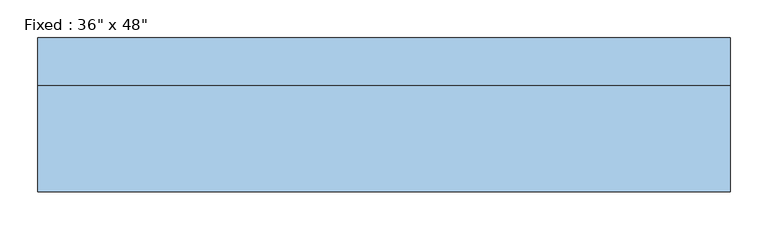
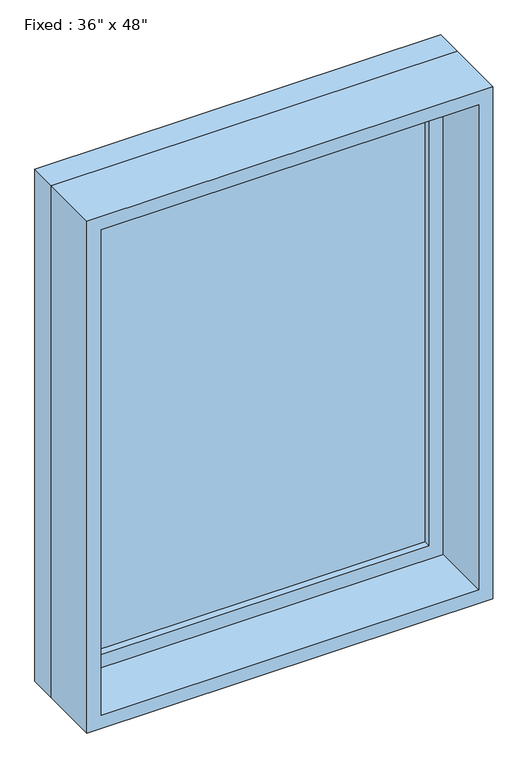
"""IFC4 building model written with IfcOpenShell, lengths in millimetres: window geometry."""

from ifc_helpers import new_model, si_unit, frame, origin, place, context, project, spatial, polyline, outline, extrude, source, transform, mapped, element, save


def window_e2841890(model_context):
    return source(origin(), model_context, "Body", "SweptSolid", [
        extrude(outline(polyline([(355.6, 53.975), (-431.8, 53.975), (-431.8, 66.675), (355.6, 66.675), (355.6, 53.975)])), frame((0.0, 0.0, 977.9), z_axis=(0.0, 0.0, 1.0), x_axis=(1.0, 0.0, 0.0)), (0.0, 0.0, 1.0), 1092.2),
        extrude(outline(polyline([(2114.55, -476.25), (933.45, -476.25), (933.45, 400.05), (2114.55, 400.05), (2114.55, -476.25)]), holes=[polyline([(2070.1, -431.8), (2070.1, 355.6), (977.9, 355.6), (977.9, -431.8), (2070.1, -431.8)])]), frame((0.0, 38.1, 0.0), z_axis=(0.0, 1.0, 0.0), x_axis=(0.0, 0.0, 1.0)), (0.0, 0.0, 1.0), 44.45),
        extrude(outline(polyline([(2133.6, -495.3), (914.4, -495.3), (914.4, 419.1), (2133.6, 419.1), (2133.6, -495.3)]), holes=[polyline([(2101.85, -463.55), (2101.85, 387.35), (946.15, 387.35), (946.15, -463.55), (2101.85, -463.55)])]), frame((0.0, -101.6, 0.0), z_axis=(0.0, 1.0, 0.0), x_axis=(0.0, 0.0, 1.0)), (0.0, 0.0, 1.0), 139.7),
        extrude(outline(polyline([(2133.6, 419.1), (2133.6, -495.3), (914.4, -495.3), (914.4, 419.1), (2133.6, 419.1)]), holes=[polyline([(2114.55, 400.05), (933.45, 400.05), (933.45, -476.25), (2114.55, -476.25), (2114.55, 400.05)])]), frame((0.0, 38.1, 0.0), z_axis=(0.0, 1.0, 0.0), x_axis=(0.0, 0.0, 1.0)), (0.0, 0.0, 1.0), 63.5),
    ])


if __name__ == "__main__":
    model = new_model("IFC4")
    model_context = context("Model", 3, world=origin())
    ifc_project = project(units=[si_unit("LENGTHUNIT", "METRE", prefix="MILLI")], contexts=[model_context])
    site = spatial("IfcSite", under=ifc_project)
    building = spatial("IfcBuilding", under=site)
    placement = place(None, origin())
    window_shape = window_e2841890(model_context)
    element("IfcWindow", 1, ObjectType="Fixed : 36\" x 48\"", at=placement, inside=building, context=model_context, shape_type="MappedRepresentation", body=[
        mapped(window_shape, transform((0.0, 0.0, 0.0), x_axis=(1.0, 0.0, 0.0), y_axis=(0.0, 1.0, 0.0), z_axis=(0.0, 0.0, 1.0))),
    ])
    save(model, "model.ifc")

# Revit data of these elements
# Type "Fixed : 36\" x 48\""
#   Type Mark = "1"
#   Construction Type Id = "GSP4R"
#   Assembly Code = "B2020100"
#   Analytic Construction = "1/8 in Pilkington single glazing"
#   Visual Light Transmittance = 0.9
#   Solar Heat Gain Coefficient = 0.78
#   Heat Transfer Coefficient (U) = 0.6496 BTU/(h·ft²·°F)
#   Height = 4' - 0"
#   Default Sill Height = 3' - 0"
#   Width = 3' - 0"
#   Window Inset = 0' - 0 3/4"
#   Define Thermal Properties by = 1
#   Glass Pane Material = Glass
#   Sash Material = Sash
#   Wall Closure = (empty or 0)
# Element 1 (IfcWindow, "Fixed : 36\" x 48\"")
#   Materials on its faces: "Sash", "Glass"
# Materials
#   "Glass": class "Glass", colour RGB 0 128 192, transparency 0.75, Description = "Soda Lime Glass", Cost = 0
#   "Sash": class "Wood", colour RGB 224 178 126, transparency 0
